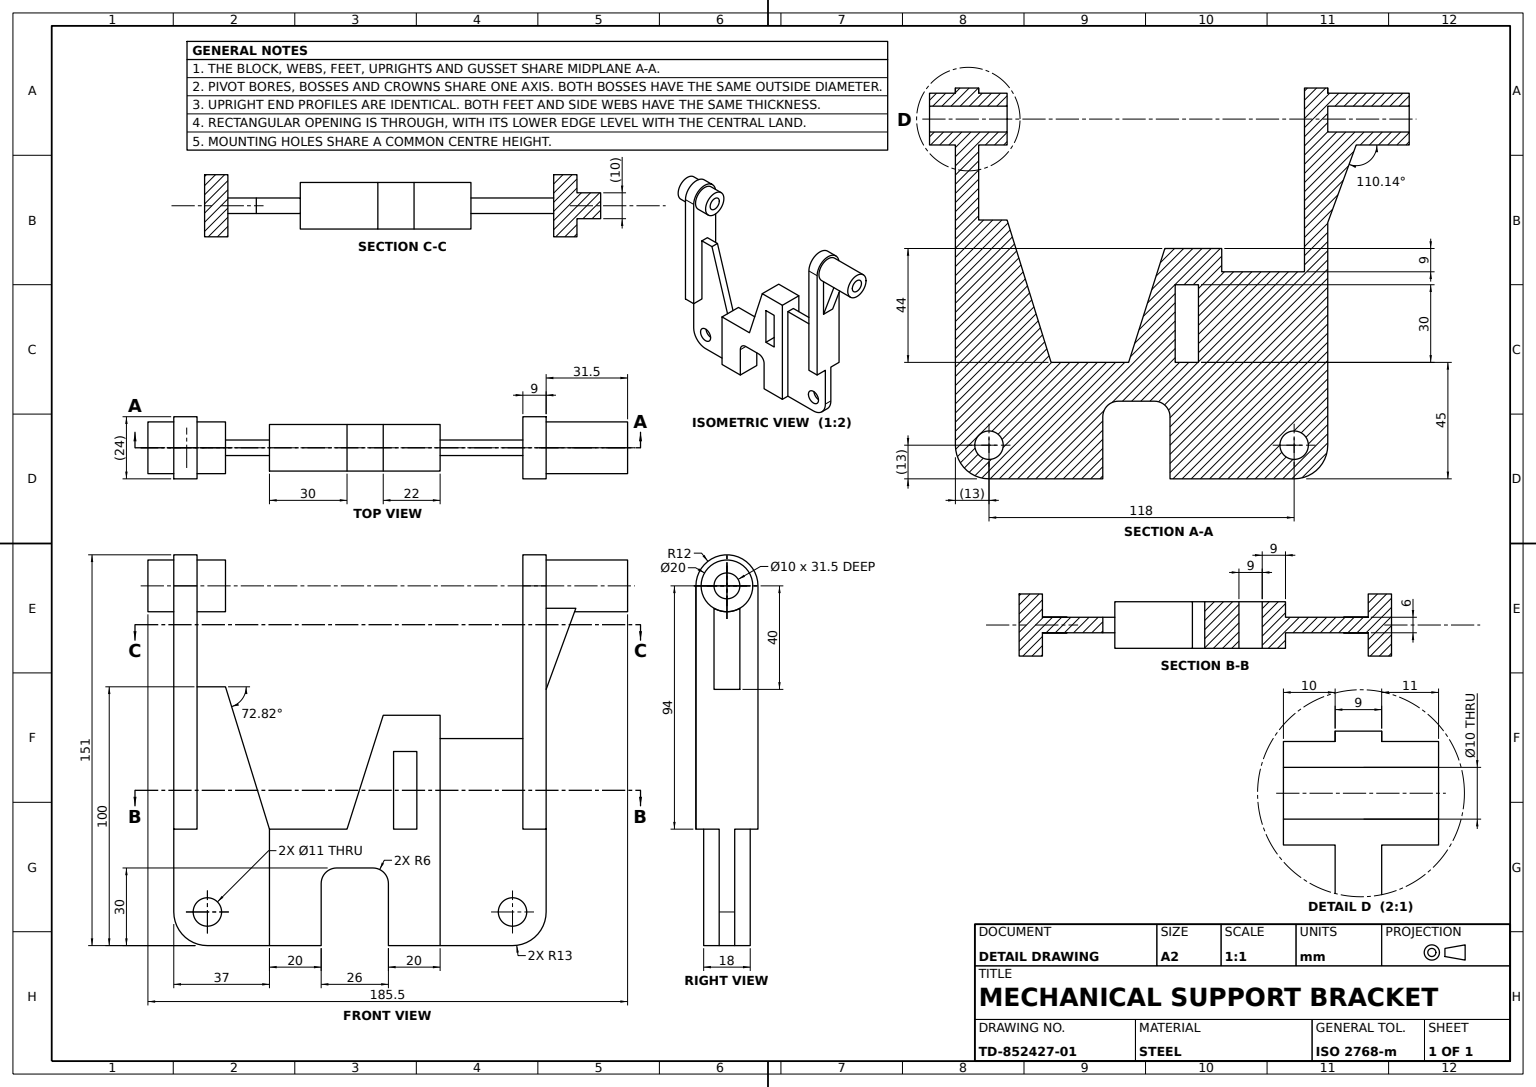
SolidWorks part; units mm, degrees
material "Plain Carbon Steel"
ref_plane "Front Plane" through (0, 0, 0) normal (0, 0, 1) x (1, 0, 0)
ref_plane "Top Plane" through (0, 0, 0) normal (0, 1, 0) x (1, 0, 0)
ref_plane "Right Plane" through (0, 0, 0) normal (1, 0, 0) x (0, 0, -1)
sketch "Base Plate Sketch" plane through (0, 0, 0) normal (0, 0, 1) x (1, 0, 0)
  line L0 (-99.3168, 0) -> (117.4332, 0) construction
  line L1 (-7, 30) -> (7, 30)
  line L2 (-13, 24) -> (-13, 0)
  line L4 (13, 24) -> (13, 0)
  line L5 (-33, 45) -> (-3, 45)
  line L6 (33, 89) -> (11, 89)
  line L8 (-33, 45) -> (-33, 0)
  line L10 (33, 89) -> (33, 0)
  line L11 (-3, 45) -> (11, 89)
  line L12 (-33, 0) -> (-13, 0)
  line L13 (13, 0) -> (33, 0)
  line L15 (15, 75) -> (24, 75)
  line L16 (15, 75) -> (15, 45)
  line L17 (15, 45) -> (24, 45)
  line L18 (24, 75) -> (24, 45)
  arc A0 (7, 30) -> (13, 24) centre (7, 24) cw
  arc A1 (-7, 30) -> (-13, 24) centre (-7, 24) ccw
  point P0 (0, 0)
  point P6 (0, 0)
  point P17 (13, 30)
  point P20 (-13, 30)
  dimension "D10" = 6
  dimension "D1" = 26
  dimension "D2" = 20
  dimension "D3" = 45
  dimension "D4" = 44
  dimension "D5" = 30
  dimension "D6" = 22
  dimension "D7" = 13
  dimension "D8" = 33
  dimension "D9" = 30
  dimension "D11" = 45
  dimension "D12" = 30
  dimension "D13" = 9
  dimension "D14" = 9
extrude "Base Plate" add sketch "Base Plate Sketch" along normal mid plane 18
sketch "Left Arm Sketch" plane through (0, 0, 0) normal (0, 0, 1) x (1, 0, 0)
  line L0 (33, 0) -> (61, 0)
  line L1 (74, 13) -> (74, 80)
  line L2 (74, 80) -> (33, 80)
  line L3 (33, 0) -> (33, 89) construction
  line L4 (33, 89) -> (11, 89) construction
  line L5 (33, 0) -> (33, 80)
  arc A0 (61, 0) -> (74, 13) centre (61, 13) ccw
  circle A1 centre (61, 13) radius 5.5
  point P11 (74, 0)
  dimension "D3" = 13
  dimension "D4" = 11
  dimension "D1" = 74
  dimension "D2" = 9
extrude "Left Arm" add sketch "Left Arm Sketch" along normal mid plane 6 contours L2 L5 L0 A0 L1
sketch "Left Arm Upright Sketch" plane through (74, 0, 0) normal (1, 0, 0) x (0, 0, -1)
  line L0 (9, 0) -> (9, 89) construction
  line L1 (-12, 45) -> (12, 45)
  line L2 (-12, 45) -> (-12, 139)
  line L4 (12, 45) -> (12, 139)
  line L6 (3, 0) -> (9, 0) construction
  line L7 (-9, 89) -> (9, 89) construction
  arc A0 (12, 139) -> (-12, 139) centre (0, 139) ccw
  dimension "D5" = 50
  dimension "D3" = 12
  dimension "D1" = 24
  dimension "D2" = 3
  dimension "D4" = 45
extrude "Left Arm Upright" add sketch "Left Arm Upright Sketch" against normal blind 9
sketch "Left Pivot Boss Sketch" plane through (74, 0, 0) normal (1, 0, 0) x (0, 0, -1)
  circle A0 centre (0, 139) radius 5
  circle A1 centre (0, 139) radius 10
  dimension "D1" = 20
  dimension "D2" = 10
extrude "Left Pivot Boss Ø20" add sketch "Left Pivot Boss Sketch" along normal blind 31.5
sketch "Left Gusset Sketch" plane through (0, 0, 0) normal (0, 0, 1) x (1, 0, 0)
  line L0 (85, 129) -> (74, 99)
  line L1 (74, 129) -> (105.5, 129) construction
  line L2 (74, 139) -> (74, 45) construction
  dimension "D1" = 11
  dimension "D2" = 30
rib "Left Gusset Rib" sketch "Left Gusset Sketch" sketch "Left Gusset Sketch" thickness 10 extrusion direction parallel to sketch draft on no parameters "D1"=10
sketch "Right Arm Sketch" plane through (0, 0, 0) normal (0, 0, 1) x (1, 0, 0)
  line L0 (-33, 0) -> (-57, 0)
  line L1 (-70, 13) -> (-70, 100)
  line L2 (-70, 100) -> (-50, 100)
  line L3 (-50, 100) -> (-33, 45)
  line L6 (-33, 45) -> (-33, 0) construction
  line L7 (-33, 45) -> (-33, 0)
  arc A0 (-57, 0) -> (-70, 13) centre (-57, 13) cw
  circle A1 centre (-57, 13) radius 5.5
  point P10 (-70, 0)
  dimension "D4" = 13
  dimension "D5" = 11
  dimension "D1" = 37
  dimension "D2" = 20
  dimension "D3" = 100
extrude "Right Arm" add sketch "Right Arm Sketch" along normal mid plane 6
sketch "Right Arm Upright Sketch" plane through (-70, 0, 0) normal (-1, 0, 0) x (0, 0, 1)
  line L0 (-3, 0) -> (-9, 0) construction
  line L1 (12, 45) -> (-12, 45)
  line L2 (12, 45) -> (12, 139)
  line L4 (-12, 45) -> (-12, 139)
  arc A1 (12, 139) -> (-12, 139) centre (0, 139) ccw
  dimension "D5" = 12
  dimension "D1" = 45
  dimension "D2" = 24
  dimension "D3" = 12
  dimension "D4" = 94
  dimension "D6" = 139
extrude "Right Arm Upright" add sketch "Right Arm Upright Sketch" against normal blind 9
sketch "Right Pivot Boss Sketch" plane through (-70, 0, 0) normal (-1, 0, 0) x (0, 0, 1)
  circle A0 centre (0, 139) radius 10
  circle A1 centre (0, 139) radius 5
  dimension "D1" = 20
  dimension "D2" = 10
extrude "Right Pivot Boss Ø20" add sketch "Right Pivot Boss Sketch" along normal blind 10 and the other way blind 20
sketch "Pivot Cut Sketch" plane through (-50, 0, 0) normal (1, 0, 0) x (0, 0, -1)
  circle A1 centre (0, 139) radius 5
  circle A2 centre (0, 139) radius 5
  dimension "D1" = 0
extrude "Pivot Cut" cut sketch "Pivot Cut Sketch" against normal blind 38
